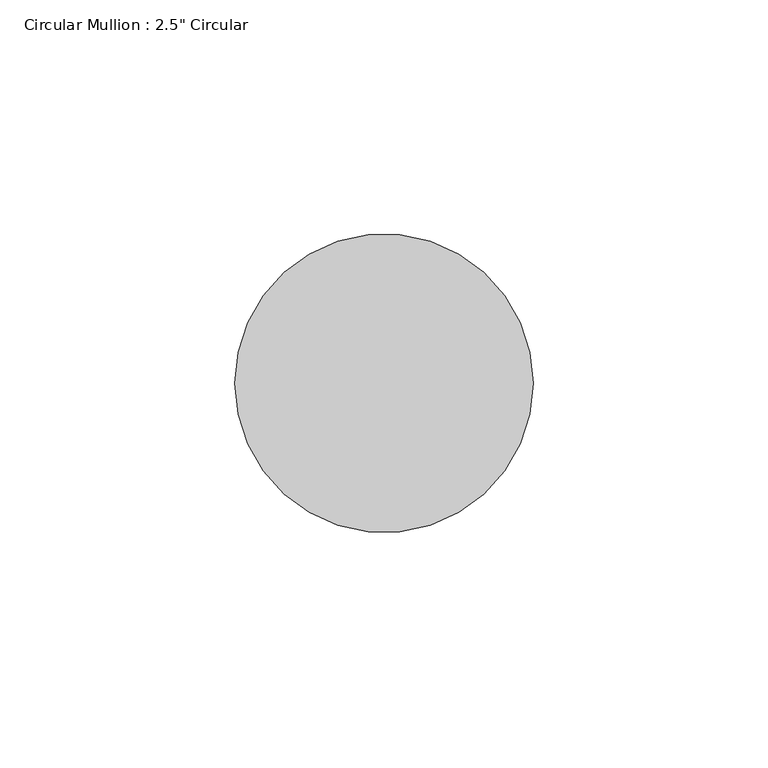
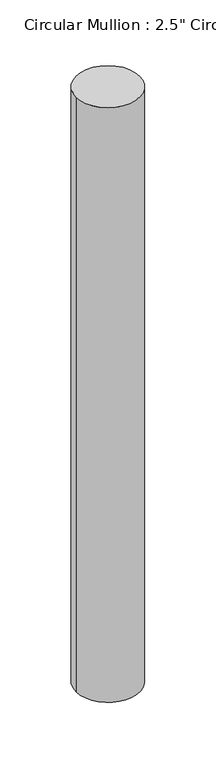
"""IFC4 building model written with IfcOpenShell, lengths in millimetres: member geometry."""

from ifc_helpers import new_model, si_unit, point, frame, origin, origin_2d, place, context, project, spatial, circle_curve, trimmed, segment, composite_curve, outline, extrude, source, transform, mapped, element, save


def member_28930b13(model_context):
    return source(origin(), model_context, "Body", "SweptSolid", [
        extrude(outline(composite_curve([segment(trimmed(circle_curve(origin_2d(), 31.75), [point((31.75, 0.0))], [point((-31.75, 0.0))], False, "CARTESIAN"), True, "CONTINUOUS"), segment(trimmed(circle_curve(origin_2d(), 31.75), [point((-31.75, 0.0))], [point((31.75, 0.0))], False, "CARTESIAN"), True, "CONTINUOUS")], self_intersect=False)), frame((0.0, 0.0, -626.5333333), z_axis=(0.0, 0.0, 1.0), x_axis=(1.0, 0.0, 0.0)), (0.0, 0.0, 1.0), 626.5333333),
    ])


if __name__ == "__main__":
    model = new_model("IFC4")
    model_context = context("Model", 3, world=origin())
    ifc_project = project(units=[si_unit("LENGTHUNIT", "METRE", prefix="MILLI")], contexts=[model_context])
    site = spatial("IfcSite", under=ifc_project)
    building = spatial("IfcBuilding", under=site)
    placement = place(None, origin())
    member_shape = member_28930b13(model_context)
    element("IfcMember", 1, ObjectType="Circular Mullion : 2.5\" Circular", at=placement, inside=building, context=model_context, shape_type="MappedRepresentation", body=[
        mapped(member_shape, transform((0.0, 0.0, 0.0), x_axis=(1.0, 0.0, 0.0), y_axis=(0.0, 1.0, 0.0), z_axis=(0.0, 0.0, 1.0))),
    ])
    save(model, "model.ifc")

# Revit data of these elements
# Type "Circular Mullion : 2.5\" Circular"
#   built-in parameter 1007350 = 0.104167 (stored number, unit not read)
# Element 1 (IfcMember, "Circular Mullion : 2.5\" Circular")
#   Materials on its faces: "Door - Frame"
# Materials
#   "Door - Frame": colour RGB 118 70 51, transparency 0, Cost = 0
